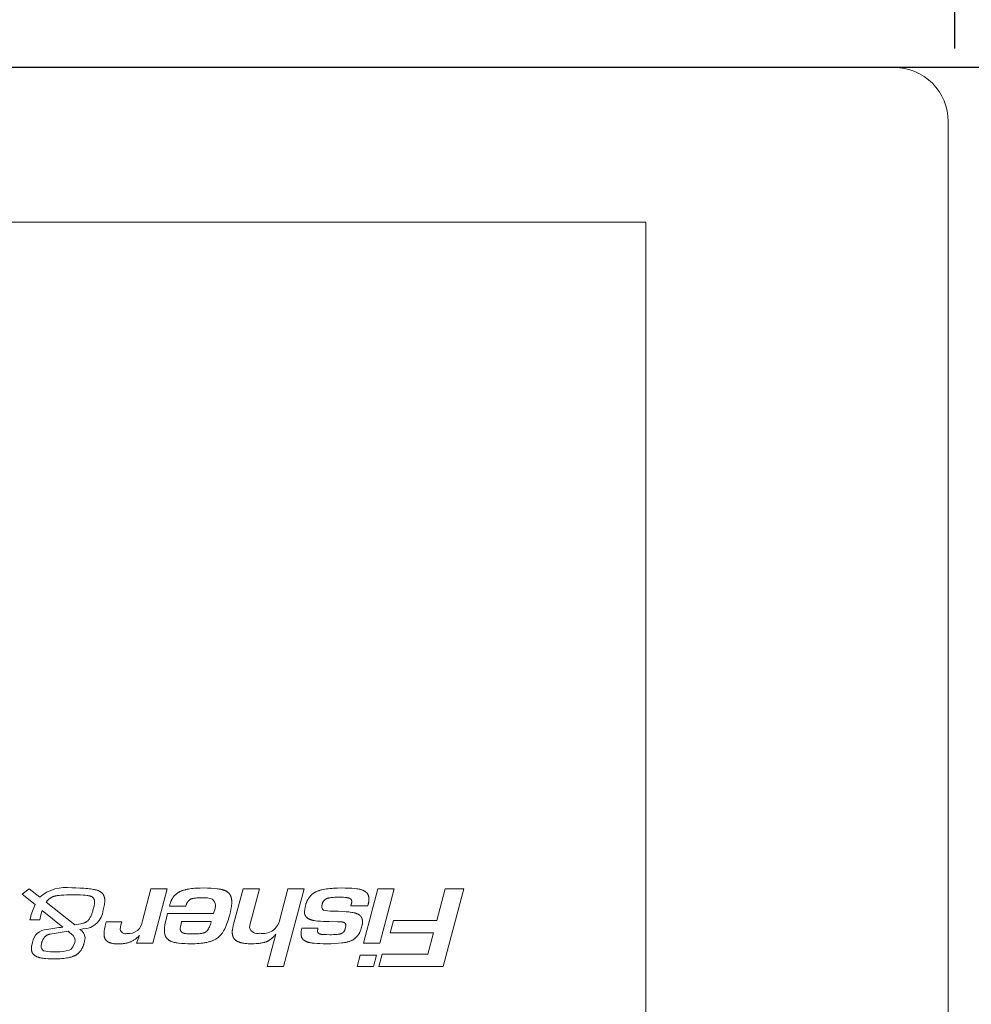
# Model space of a CAD drawing. Units: inches. Extents: x -1198 to -69, y -512 to 437.
# Tile 12 of 50: x -948.245 to -945.108, y 182.142 to 185.385. Entities that reach past the tile are written whole.
import ezdxf

# ---------------------------------------------------------------- set-up
doc = ezdxf.new("R2010")
doc.units = ezdxf.units.IN
doc.header["$MEASUREMENT"] = 0
for name, color, linetype, lineweight in [('0_Pen_No__7', 7, 'Continuous', 18), ('A-ANNO-DIMS', 2, 'Continuous', 18), ('A-EQPM', 60, 'Continuous', 18), ('A-FLOR-CASE', 7, 'Continuous', 25)]:
    doc.layers.add(name, color=color, linetype=linetype, lineweight=lineweight)
doc.styles.get("Standard").update_dxf_attribs({"font": 'arial.ttf'})
doc.dimstyles.get("Standard").update_dxf_attribs({"dimtxt": 6, "dimasz": 6, "dimexe": 0.18, "dimexo": 0.0625, "dimgap": 0.09, "dimtad": 0, "dimtih": 1, "dimtoh": 1, "dimdec": 0, "dimzin": 0, "dimdsep": 46, "dimlunit": 4, "dimtxsty": 'Standard', "dimblk": 'OBLIQUE', "dimcen": 0.09, "dimadec": 0, "dimazin": 0, "dimtfac": 1, "dimtdec": 0, "dimtofl": 0, "dimtmove": 0, "dimatfit": 3, "dimfxl": 1, "dimtolj": 1, "dimtzin": 0, "dimarcsym": 0})

# ---------------------------------------------------------------- blocks, each defined once
blk = doc.blocks.new('new block')
at = {"layer": '0_Pen_No__7'}
for p, q in [((-318.452, 68.7), (-316.721, 75.2)), ((-316.721, 75.2), (-311.349, 75.2)), ((-311.349, 75.2), (-311.629, 74.168)), ((-311.16, 74.266), (-310.904, 75.2)), ((-310.904, 75.2), (-309.527, 75.2)), ((-309.527, 75.2), (-309.782, 74.266)), ((-305.104, 68.7), (-303.373, 75.2)), ((-303.373, 75.2), (-301.997, 75.2)), ((-301.997, 75.2), (-302.715, 72.502)), ((-315.442, 74.168), (-315.906, 72.403)), ((-311.629, 74.168), (-315.442, 74.168)), ((-309.782, 74.266), (-311.16, 74.266)), ((-312.634, 68.7), (-311.429, 73.251)), ((-311.429, 73.251), (-310.05, 73.251)), ((-310.05, 73.251), (-311.257, 68.7)), ((-293.639, 68.7), (-292.433, 73.251)), ((-292.433, 73.251), (-291.056, 73.251)), ((-291.056, 73.251), (-291.311, 72.618)), ((-286.771, 72.786), (-286.716, 73.132)), ((-285.755, 72.627), (-285.462, 72.368)), ((-315.906, 72.403), (-312.288, 72.403)), ((-312.288, 72.403), (-312.567, 71.371)), ((-306.237, 72.004), (-306.225, 72.092)), ((-304.908, 72.004), (-306.237, 72.004)), ((-306.225, 72.092), (-306.213, 72.219)), ((-300.571, 71.634), (-300.522, 71.955)), ((-299.158, 71.789), (-299.974, 68.7)), ((-294.784, 71.634), (-294.723, 72.033)), ((-289.824, 71.488), (-289.753, 71.731)), ((-289.753, 71.731), (-289.691, 72.102)), ((-288.448, 71.819), (-288.533, 71.488)), ((-286.562, 72.059), (-286.329, 72.102)), ((-283.509, 69.837), (-285.894, 71.738)), ((-285.462, 72.368), (-285.335, 72.264)), ((-284.895, 71.907), (-283.174, 70.513)), ((-316.186, 71.371), (-316.892, 68.7)), ((-312.567, 71.371), (-316.186, 71.371)), ((-303.045, 71.283), (-303.727, 68.7)), ((-301.351, 68.7), (-300.571, 71.634)), ((-297.319, 71.458), (-294.833, 71.458)), ((-294.833, 71.458), (-294.784, 71.634)), ((-293.566, 71.146), (-293.663, 70.776)), ((-291.555, 71.379), (-292.26, 68.7)), ((-288.533, 71.488), (-289.824, 71.488)), ((-283.174, 70.513), (-283.064, 70.877)), ((-283.064, 70.877), (-282.962, 71.312)), ((-282.962, 71.312), (-282.141, 71.312)), ((-282.242, 70.858), (-282.564, 70.016)), ((-282.174, 71.152), (-282.242, 70.858)), ((-282.141, 71.312), (-282.174, 71.152)), ((-310.452, 70.006), (-310.417, 70.134)), ((-310.417, 70.134), (-309.003, 70.134)), ((-309.003, 70.134), (-309.04, 69.986)), ((-306.725, 70.503), (-307.261, 70.58)), ((-305.117, 70.62), (-305.202, 70.114)), ((-297.514, 70.776), (-297.561, 70.601)), ((-293.663, 70.776), (-297.514, 70.776)), ((-295.187, 70.152), (-293.822, 70.152)), ((-293.846, 70.065), (-293.858, 70.016)), ((-293.822, 70.152), (-293.846, 70.065)), ((-288.382, 70.016), (-288.272, 70.467)), ((-288.405, 69.686), (-288.382, 70.016)), ((-282.063, 68.7), (-282.973, 69.42)), ((-282.564, 70.016), (-281.486, 69.163)), ((-316.892, 68.7), (-318.452, 68.7)), ((-311.257, 68.7), (-312.634, 68.7)), ((-303.727, 68.7), (-305.104, 68.7)), ((-299.974, 68.7), (-301.351, 68.7)), ((-292.26, 68.7), (-293.639, 68.7)), ((-281.486, 69.163), (-282.063, 68.7))]:
    blk.add_line(p, q, dxfattribs=at)
blk.add_lwpolyline([(-354.492, 596.906), (481.176, 596.906, -0.414214), (485.681, 592.401), (485.681, 99.109), (486.244, 99.109), (486.244, 95.73), (485.681, 95.73), (485.681, 4.505, -0.414214), (481.176, 0), (-354.492, 0, -0.414214), (-358.997, 4.505), (-358.997, 95.73), (-359.56, 95.73), (-359.56, 99.109), (-358.997, 99.109), (-358.997, 592.401, -0.414214)], format="xyb", close=True, dxfattribs=at)
blk.add_lwpolyline([(-333.701, 12.952), (460.296, 12.952), (460.296, 570.439), (-333.701, 570.439)], close=True, dxfattribs=at)
for points in [[(-286.716, 73.132), (-286.69, 73.224), (-286.662, 73.317), (-286.646, 73.362), (-286.63, 73.408), (-286.613, 73.453), (-286.595, 73.498), (-286.577, 73.543), (-286.557, 73.587), (-286.536, 73.63), (-286.514, 73.673), (-286.492, 73.716), (-286.468, 73.757), (-286.443, 73.799), (-286.417, 73.839), (-286.394, 73.873), (-286.37, 73.906), (-286.345, 73.938), (-286.32, 73.97), (-286.294, 74.001), (-286.266, 74.031), (-286.238, 74.06), (-286.209, 74.089), (-286.181, 74.115), (-286.152, 74.14), (-286.122, 74.164), (-286.091, 74.187), (-286.06, 74.209), (-286.028, 74.23), (-285.996, 74.25), (-285.963, 74.269), (-285.924, 74.29), (-285.885, 74.309), (-285.846, 74.327), (-285.806, 74.344), (-285.765, 74.36), (-285.724, 74.375), (-285.683, 74.389), (-285.641, 74.402), (-285.59, 74.417), (-285.538, 74.431), (-285.486, 74.444), (-285.434, 74.456), (-285.329, 74.478), (-285.223, 74.496), (-285.084, 74.517), (-284.943, 74.534), (-284.803, 74.547), (-284.662, 74.557), (-284.521, 74.564), (-284.379, 74.568), (-284.097, 74.572)], [(-284.097, 74.572), (-283.885, 74.569), (-283.673, 74.56), (-283.461, 74.545), (-283.355, 74.535), (-283.249, 74.523), (-283.177, 74.513), (-283.105, 74.502), (-283.033, 74.489), (-282.997, 74.481), (-282.962, 74.473), (-282.926, 74.464), (-282.891, 74.455), (-282.856, 74.444), (-282.821, 74.433), (-282.787, 74.42), (-282.753, 74.407), (-282.719, 74.393), (-282.686, 74.377), (-282.662, 74.365), (-282.639, 74.353), (-282.616, 74.34), (-282.594, 74.326), (-282.572, 74.312), (-282.55, 74.297), (-282.529, 74.282), (-282.508, 74.266), (-282.488, 74.249), (-282.478, 74.24), (-282.469, 74.232), (-282.459, 74.223), (-282.45, 74.214), (-282.441, 74.204), (-282.432, 74.195), (-282.423, 74.186), (-282.415, 74.176), (-282.407, 74.166), (-282.399, 74.156), (-282.391, 74.146), (-282.383, 74.135), (-282.376, 74.125), (-282.369, 74.114), (-282.362, 74.103), (-282.355, 74.091), (-282.349, 74.08), (-282.343, 74.068), (-282.337, 74.056), (-282.331, 74.044), (-282.326, 74.032), (-282.32, 74.02), (-282.315, 74.007), (-282.311, 73.995), (-282.306, 73.982), (-282.302, 73.969), (-282.298, 73.956), (-282.294, 73.943), (-282.291, 73.93), (-282.288, 73.917), (-282.282, 73.891), (-282.277, 73.864), (-282.273, 73.837), (-282.269, 73.81), (-282.267, 73.782), (-282.265, 73.755), (-282.264, 73.728), (-282.263, 73.701), (-282.263, 73.669), (-282.265, 73.638), (-282.267, 73.606), (-282.269, 73.575), (-282.273, 73.544), (-282.277, 73.513), (-282.282, 73.482), (-282.287, 73.451), (-282.299, 73.39), (-282.312, 73.329), (-282.342, 73.207)], [(-291.311, 72.618), (-291.264, 72.662), (-291.217, 72.706), (-291.168, 72.749), (-291.119, 72.792), (-291.069, 72.833), (-291.018, 72.873), (-290.966, 72.911), (-290.913, 72.949), (-290.866, 72.98), (-290.819, 73.011), (-290.771, 73.04), (-290.722, 73.068), (-290.673, 73.094), (-290.623, 73.119), (-290.572, 73.142), (-290.521, 73.164), (-290.468, 73.184), (-290.414, 73.203), (-290.359, 73.219), (-290.304, 73.235), (-290.249, 73.248), (-290.193, 73.26), (-290.137, 73.271), (-290.081, 73.281), (-290.017, 73.29), (-289.953, 73.298), (-289.889, 73.304), (-289.825, 73.31), (-289.755, 73.314), (-289.685, 73.317), (-289.545, 73.319), (-289.472, 73.319), (-289.4, 73.317), (-289.327, 73.313), (-289.255, 73.307), (-289.192, 73.301), (-289.13, 73.293), (-289.068, 73.283), (-289.006, 73.271), (-288.956, 73.26), (-288.907, 73.247), (-288.883, 73.24), (-288.859, 73.233), (-288.835, 73.225), (-288.811, 73.216), (-288.787, 73.207), (-288.764, 73.197), (-288.741, 73.187), (-288.718, 73.176), (-288.696, 73.164), (-288.674, 73.151), (-288.663, 73.145), (-288.653, 73.138), (-288.642, 73.131), (-288.632, 73.124), (-288.615, 73.111), (-288.598, 73.098), (-288.581, 73.085), (-288.565, 73.07), (-288.549, 73.056), (-288.534, 73.041), (-288.52, 73.025), (-288.505, 73.009), (-288.492, 72.992), (-288.478, 72.975), (-288.466, 72.958), (-288.454, 72.94), (-288.442, 72.922), (-288.432, 72.904), (-288.422, 72.885), (-288.412, 72.866), (-288.407, 72.855), (-288.402, 72.844), (-288.397, 72.832), (-288.393, 72.821), (-288.389, 72.81), (-288.385, 72.798), (-288.381, 72.786), (-288.377, 72.775), (-288.37, 72.751), (-288.364, 72.727), (-288.359, 72.703), (-288.355, 72.679), (-288.351, 72.654), (-288.347, 72.63), (-288.345, 72.605), (-288.343, 72.58), (-288.341, 72.556), (-288.34, 72.531), (-288.339, 72.481), (-288.34, 72.439), (-288.341, 72.396), (-288.344, 72.354), (-288.347, 72.312), (-288.352, 72.27), (-288.357, 72.229), (-288.363, 72.187), (-288.37, 72.145), (-288.386, 72.063), (-288.405, 71.981), (-288.426, 71.9), (-288.448, 71.819)], [(-285.335, 72.264), (-283.828, 72.5), (-283.806, 72.504), (-283.784, 72.508), (-283.762, 72.514), (-283.739, 72.519), (-283.717, 72.526), (-283.695, 72.533), (-283.673, 72.541), (-283.652, 72.549), (-283.631, 72.558), (-283.609, 72.567), (-283.59, 72.577), (-283.572, 72.587), (-283.553, 72.597), (-283.535, 72.608), (-283.517, 72.62), (-283.5, 72.632), (-283.483, 72.644), (-283.466, 72.657), (-283.45, 72.67), (-283.435, 72.684), (-283.42, 72.697), (-283.405, 72.712), (-283.391, 72.726), (-283.377, 72.741), (-283.364, 72.756), (-283.351, 72.772), (-283.338, 72.787), (-283.326, 72.804), (-283.313, 72.82), (-283.302, 72.837), (-283.29, 72.853), (-283.279, 72.871), (-283.268, 72.888), (-283.258, 72.905), (-283.248, 72.923), (-283.239, 72.94), (-283.22, 72.976), (-283.204, 73.012), (-283.188, 73.049), (-283.173, 73.086), (-283.159, 73.123), (-283.146, 73.161), (-283.134, 73.199), (-283.124, 73.235), (-283.115, 73.27), (-283.097, 73.342), (-283.082, 73.414), (-283.068, 73.487)], [(-309.904, 71.926), (-309.878, 72.017), (-309.864, 72.062), (-309.849, 72.107), (-309.833, 72.152), (-309.816, 72.196), (-309.798, 72.24), (-309.78, 72.283), (-309.76, 72.326), (-309.739, 72.369), (-309.717, 72.411), (-309.694, 72.452), (-309.67, 72.493), (-309.645, 72.533), (-309.618, 72.572), (-309.591, 72.61), (-309.566, 72.643), (-309.54, 72.676), (-309.512, 72.707), (-309.484, 72.738), (-309.455, 72.768), (-309.426, 72.797), (-309.395, 72.825), (-309.363, 72.852), (-309.331, 72.878), (-309.298, 72.902), (-309.265, 72.926), (-309.23, 72.948), (-309.196, 72.969), (-309.16, 72.99), (-309.124, 73.009), (-309.087, 73.027), (-309.039, 73.05), (-308.989, 73.071), (-308.939, 73.091), (-308.888, 73.108), (-308.837, 73.125), (-308.785, 73.14), (-308.732, 73.154), (-308.68, 73.167), (-308.627, 73.179), (-308.573, 73.19), (-308.466, 73.209), (-308.359, 73.225), (-308.251, 73.239), (-307.955, 73.271), (-307.661, 73.292), (-307.323, 73.305), (-306.956, 73.31), (-306.678, 73.308), (-306.4, 73.299), (-306.169, 73.285), (-305.939, 73.266), (-305.777, 73.248), (-305.696, 73.237), (-305.615, 73.224), (-305.575, 73.216), (-305.535, 73.207), (-305.496, 73.198), (-305.456, 73.188), (-305.416, 73.176), (-305.377, 73.164), (-305.338, 73.15), (-305.299, 73.135), (-305.274, 73.124), (-305.249, 73.113), (-305.224, 73.102), (-305.199, 73.09), (-305.175, 73.077), (-305.151, 73.063), (-305.128, 73.049), (-305.105, 73.034), (-305.094, 73.026), (-305.083, 73.019), (-305.072, 73.01), (-305.062, 73.002), (-305.051, 72.994), (-305.041, 72.985), (-305.031, 72.976), (-305.021, 72.967), (-305.011, 72.958), (-305.002, 72.949), (-304.993, 72.939), (-304.984, 72.929), (-304.975, 72.919), (-304.967, 72.909), (-304.959, 72.899), (-304.951, 72.888), (-304.944, 72.877), (-304.937, 72.866), (-304.93, 72.855), (-304.923, 72.844), (-304.917, 72.832), (-304.911, 72.821), (-304.905, 72.809), (-304.899, 72.797), (-304.894, 72.785), (-304.889, 72.772), (-304.884, 72.76), (-304.88, 72.747), (-304.875, 72.735), (-304.871, 72.722), (-304.868, 72.709), (-304.864, 72.696), (-304.861, 72.683), (-304.858, 72.67), (-304.852, 72.643), (-304.847, 72.616), (-304.843, 72.589), (-304.84, 72.562), (-304.838, 72.535), (-304.837, 72.508), (-304.836, 72.481), (-304.836, 72.45), (-304.836, 72.42), (-304.838, 72.389), (-304.84, 72.359), (-304.843, 72.329), (-304.847, 72.299), (-304.852, 72.269), (-304.856, 72.239), (-304.867, 72.18), (-304.88, 72.121), (-304.908, 72.004)], [(-307.236, 72.55), (-307.388, 72.549), (-307.54, 72.544), (-307.693, 72.536), (-307.846, 72.525), (-307.939, 72.516), (-307.986, 72.511), (-308.009, 72.507), (-308.032, 72.503), (-308.055, 72.499), (-308.078, 72.494), (-308.101, 72.489), (-308.123, 72.483), (-308.145, 72.476), (-308.167, 72.469), (-308.189, 72.461), (-308.2, 72.457), (-308.211, 72.452), (-308.224, 72.446), (-308.238, 72.44), (-308.251, 72.433), (-308.264, 72.426), (-308.277, 72.418), (-308.29, 72.411), (-308.302, 72.403), (-308.315, 72.394), (-308.327, 72.386), (-308.338, 72.377), (-308.35, 72.367), (-308.361, 72.358), (-308.372, 72.348), (-308.383, 72.337), (-308.393, 72.326), (-308.403, 72.315), (-308.413, 72.304), (-308.422, 72.292), (-308.431, 72.28), (-308.439, 72.267), (-308.447, 72.255), (-308.455, 72.242), (-308.463, 72.228), (-308.47, 72.215), (-308.477, 72.201), (-308.483, 72.188), (-308.489, 72.174), (-308.495, 72.159), (-308.5, 72.145), (-308.505, 72.131), (-308.51, 72.117), (-308.515, 72.102), (-308.522, 72.075), (-308.529, 72.048), (-308.535, 72.02), (-308.568, 71.844), (-308.572, 71.825), (-308.575, 71.807), (-308.577, 71.788), (-308.578, 71.769), (-308.578, 71.75), (-308.577, 71.736), (-308.576, 71.721), (-308.574, 71.711), (-308.572, 71.701), (-308.57, 71.691), (-308.567, 71.681), (-308.564, 71.671), (-308.561, 71.662), (-308.557, 71.652), (-308.552, 71.643), (-308.548, 71.634), (-308.543, 71.625), (-308.538, 71.616), (-308.532, 71.608), (-308.526, 71.6), (-308.516, 71.589), (-308.508, 71.58), (-308.499, 71.572), (-308.489, 71.563), (-308.478, 71.556), (-308.467, 71.549), (-308.455, 71.542), (-308.444, 71.536), (-308.431, 71.531), (-308.413, 71.523), (-308.4, 71.519), (-308.387, 71.514), (-308.374, 71.511), (-308.36, 71.507), (-308.347, 71.504), (-308.32, 71.498), (-308.294, 71.493), (-308.268, 71.488), (-308.243, 71.484), (-308.217, 71.48), (-308.166, 71.474), (-308.115, 71.47), (-308.064, 71.466), (-307.913, 71.461), (-307.2, 71.448)], [(-306.213, 72.219), (-306.213, 72.23), (-306.213, 72.242), (-306.214, 72.253), (-306.215, 72.265), (-306.217, 72.277), (-306.219, 72.288), (-306.221, 72.3), (-306.224, 72.311), (-306.227, 72.322), (-306.23, 72.333), (-306.234, 72.344), (-306.239, 72.354), (-306.244, 72.365), (-306.249, 72.375), (-306.255, 72.384), (-306.261, 72.394), (-306.268, 72.402), (-306.275, 72.411), (-306.283, 72.419), (-306.291, 72.426), (-306.299, 72.433), (-306.308, 72.44), (-306.317, 72.447), (-306.326, 72.453), (-306.336, 72.459), (-306.346, 72.465), (-306.356, 72.47), (-306.366, 72.475), (-306.376, 72.48), (-306.387, 72.484), (-306.397, 72.488), (-306.408, 72.492), (-306.427, 72.498), (-306.445, 72.504), (-306.464, 72.509), (-306.483, 72.513), (-306.502, 72.517), (-306.521, 72.52), (-306.54, 72.523), (-306.559, 72.526), (-306.597, 72.529), (-306.635, 72.532), (-306.974, 72.546), (-307.236, 72.55)], [(-302.715, 72.502), (-302.674, 72.555), (-302.631, 72.607), (-302.588, 72.659), (-302.542, 72.709), (-302.495, 72.757), (-302.447, 72.804), (-302.422, 72.827), (-302.396, 72.85), (-302.371, 72.872), (-302.345, 72.893), (-302.321, 72.912), (-302.298, 72.93), (-302.274, 72.947), (-302.249, 72.965), (-302.225, 72.981), (-302.2, 72.998), (-302.175, 73.014), (-302.149, 73.029), (-302.124, 73.044), (-302.098, 73.059), (-302.072, 73.073), (-302.045, 73.086), (-302.018, 73.099), (-301.991, 73.112), (-301.964, 73.124), (-301.937, 73.135), (-301.905, 73.147), (-301.873, 73.159), (-301.841, 73.17), (-301.809, 73.181), (-301.776, 73.191), (-301.743, 73.2), (-301.677, 73.217), (-301.611, 73.231), (-301.544, 73.244), (-301.476, 73.256), (-301.409, 73.266), (-301.327, 73.277), (-301.244, 73.286), (-301.162, 73.293), (-301.079, 73.299), (-300.893, 73.307), (-300.706, 73.31), (-300.505, 73.307), (-300.404, 73.302), (-300.304, 73.296), (-300.218, 73.288), (-300.133, 73.279), (-300.048, 73.267), (-299.963, 73.254), (-299.897, 73.241), (-299.833, 73.227), (-299.8, 73.22), (-299.768, 73.211), (-299.736, 73.202), (-299.705, 73.193), (-299.673, 73.182), (-299.642, 73.171), (-299.611, 73.159), (-299.581, 73.146), (-299.551, 73.133), (-299.521, 73.118), (-299.492, 73.102), (-299.477, 73.094), (-299.463, 73.085), (-299.441, 73.071), (-299.419, 73.057), (-299.397, 73.041), (-299.376, 73.025), (-299.356, 73.009), (-299.335, 72.992), (-299.316, 72.974), (-299.297, 72.955), (-299.278, 72.936), (-299.261, 72.917), (-299.244, 72.897), (-299.236, 72.887), (-299.228, 72.876), (-299.22, 72.866), (-299.212, 72.855), (-299.205, 72.844), (-299.197, 72.833), (-299.19, 72.822), (-299.184, 72.811), (-299.177, 72.8), (-299.171, 72.788), (-299.164, 72.776), (-299.158, 72.763), (-299.152, 72.751), (-299.146, 72.738), (-299.14, 72.725), (-299.135, 72.712), (-299.13, 72.698), (-299.125, 72.685), (-299.121, 72.672), (-299.116, 72.658), (-299.109, 72.631), (-299.101, 72.603), (-299.095, 72.575), (-299.09, 72.547), (-299.085, 72.518), (-299.082, 72.49), (-299.079, 72.461), (-299.076, 72.433), (-299.075, 72.404), (-299.074, 72.375), (-299.073, 72.346), (-299.073, 72.311), (-299.074, 72.275), (-299.076, 72.239), (-299.079, 72.204), (-299.082, 72.169), (-299.086, 72.134), (-299.091, 72.099), (-299.096, 72.064), (-299.109, 71.994), (-299.123, 71.925), (-299.14, 71.857), (-299.158, 71.789)], [(-298.842, 70.97), (-298.801, 71.12), (-298.757, 71.27), (-298.71, 71.418), (-298.659, 71.565), (-298.603, 71.711), (-298.574, 71.783), (-298.543, 71.854), (-298.511, 71.925), (-298.477, 71.995), (-298.442, 72.064), (-298.406, 72.133), (-298.376, 72.186), (-298.345, 72.239), (-298.313, 72.292), (-298.28, 72.343), (-298.246, 72.394), (-298.211, 72.444), (-298.174, 72.493), (-298.135, 72.54), (-298.101, 72.581), (-298.066, 72.62), (-298.029, 72.659), (-297.992, 72.696), (-297.953, 72.733), (-297.913, 72.767), (-297.893, 72.784), (-297.872, 72.801), (-297.851, 72.817), (-297.83, 72.833), (-297.808, 72.849), (-297.785, 72.864), (-297.763, 72.879), (-297.739, 72.894), (-297.692, 72.922), (-297.645, 72.948), (-297.596, 72.974), (-297.546, 72.997), (-297.496, 73.02), (-297.446, 73.041), (-297.385, 73.064), (-297.324, 73.086), (-297.263, 73.107), (-297.201, 73.126), (-297.139, 73.144), (-297.076, 73.16), (-296.95, 73.19), (-296.869, 73.207), (-296.787, 73.222), (-296.705, 73.236), (-296.622, 73.249), (-296.457, 73.27), (-296.291, 73.286), (-296.125, 73.297), (-295.958, 73.305), (-295.625, 73.31)], [(-295.807, 72.492), (-295.973, 72.49), (-296.056, 72.488), (-296.139, 72.484), (-296.222, 72.478), (-296.304, 72.47), (-296.386, 72.46), (-296.468, 72.448), (-296.526, 72.437), (-296.585, 72.424), (-296.614, 72.417), (-296.643, 72.41), (-296.671, 72.401), (-296.7, 72.392), (-296.722, 72.385), (-296.744, 72.377), (-296.765, 72.369), (-296.787, 72.36), (-296.797, 72.355), (-296.808, 72.35), (-296.818, 72.345), (-296.828, 72.339), (-296.838, 72.334), (-296.848, 72.328), (-296.858, 72.322), (-296.867, 72.315), (-296.876, 72.309), (-296.885, 72.303), (-296.893, 72.296), (-296.902, 72.29), (-296.91, 72.283), (-296.918, 72.275), (-296.926, 72.268), (-296.934, 72.261), (-296.941, 72.253), (-296.949, 72.245), (-296.964, 72.229), (-296.978, 72.213), (-296.992, 72.196), (-297.008, 72.175), (-297.024, 72.153), (-297.04, 72.13), (-297.054, 72.107), (-297.069, 72.084), (-297.082, 72.061), (-297.109, 72.013), (-297.126, 71.98), (-297.142, 71.947), (-297.158, 71.913), (-297.173, 71.879), (-297.201, 71.811), (-297.228, 71.741), (-297.253, 71.671), (-297.276, 71.6), (-297.319, 71.458)], [(-294.723, 72.033), (-294.723, 72.048), (-294.724, 72.063), (-294.725, 72.079), (-294.726, 72.094), (-294.728, 72.11), (-294.73, 72.125), (-294.732, 72.14), (-294.736, 72.155), (-294.739, 72.17), (-294.743, 72.185), (-294.748, 72.2), (-294.753, 72.214), (-294.759, 72.228), (-294.766, 72.242), (-294.773, 72.255), (-294.781, 72.268), (-294.789, 72.279), (-294.797, 72.29), (-294.806, 72.3), (-294.815, 72.31), (-294.825, 72.32), (-294.835, 72.329), (-294.846, 72.338), (-294.857, 72.347), (-294.868, 72.355), (-294.88, 72.363), (-294.891, 72.37), (-294.904, 72.377), (-294.916, 72.384), (-294.928, 72.391), (-294.941, 72.397), (-294.954, 72.403), (-294.963, 72.407), (-294.973, 72.411), (-294.992, 72.418), (-295.012, 72.425), (-295.032, 72.431), (-295.052, 72.436), (-295.072, 72.441), (-295.092, 72.445), (-295.113, 72.449), (-295.133, 72.453), (-295.154, 72.456), (-295.195, 72.461), (-295.277, 72.469), (-295.41, 72.479), (-295.542, 72.486), (-295.675, 72.491), (-295.807, 72.492)], [(-295.625, 73.31), (-295.36, 73.306), (-295.094, 73.296), (-294.828, 73.278), (-294.562, 73.251), (-294.474, 73.241), (-294.386, 73.229), (-294.299, 73.214), (-294.255, 73.205), (-294.212, 73.196), (-294.169, 73.186), (-294.127, 73.174), (-294.085, 73.161), (-294.043, 73.147), (-294.002, 73.132), (-293.982, 73.124), (-293.962, 73.115), (-293.942, 73.106), (-293.922, 73.097), (-293.902, 73.087), (-293.882, 73.077), (-293.855, 73.062), (-293.827, 73.045), (-293.8, 73.028), (-293.774, 73.01), (-293.748, 72.991), (-293.723, 72.972), (-293.699, 72.951), (-293.675, 72.93), (-293.652, 72.908), (-293.641, 72.897), (-293.63, 72.886), (-293.619, 72.874), (-293.608, 72.862), (-293.598, 72.85), (-293.588, 72.838), (-293.578, 72.826), (-293.568, 72.813), (-293.559, 72.801), (-293.55, 72.788), (-293.541, 72.775), (-293.533, 72.762), (-293.525, 72.748), (-293.517, 72.735), (-293.508, 72.719), (-293.5, 72.704), (-293.492, 72.688), (-293.484, 72.672), (-293.477, 72.655), (-293.47, 72.639), (-293.464, 72.622), (-293.458, 72.606), (-293.452, 72.589), (-293.447, 72.572), (-293.442, 72.555), (-293.437, 72.537), (-293.432, 72.52), (-293.428, 72.503), (-293.42, 72.467), (-293.414, 72.432), (-293.409, 72.396), (-293.404, 72.36), (-293.401, 72.324), (-293.398, 72.288), (-293.396, 72.251), (-293.395, 72.215), (-293.395, 72.179), (-293.396, 72.122), (-293.398, 72.065), (-293.402, 72.009), (-293.407, 71.953), (-293.413, 71.897), (-293.42, 71.842), (-293.437, 71.731), (-293.464, 71.584), (-293.495, 71.437), (-293.529, 71.291), (-293.566, 71.146)], [(-307.261, 70.58), (-307.93, 70.588), (-308.264, 70.602), (-308.598, 70.625), (-308.835, 70.648), (-308.954, 70.663), (-309.072, 70.68), (-309.159, 70.695), (-309.246, 70.712), (-309.29, 70.722), (-309.333, 70.732), (-309.375, 70.744), (-309.418, 70.757), (-309.45, 70.767), (-309.481, 70.779), (-309.513, 70.791), (-309.543, 70.804), (-309.574, 70.818), (-309.604, 70.833), (-309.619, 70.841), (-309.634, 70.849), (-309.648, 70.857), (-309.663, 70.866), (-309.675, 70.874), (-309.687, 70.882), (-309.699, 70.89), (-309.711, 70.898), (-309.723, 70.907), (-309.734, 70.916), (-309.746, 70.925), (-309.757, 70.934), (-309.768, 70.944), (-309.778, 70.954), (-309.789, 70.964), (-309.799, 70.974), (-309.809, 70.984), (-309.819, 70.995), (-309.828, 71.006), (-309.837, 71.017), (-309.846, 71.029), (-309.854, 71.04), (-309.862, 71.052), (-309.87, 71.064), (-309.877, 71.076), (-309.884, 71.088), (-309.891, 71.101), (-309.898, 71.113), (-309.904, 71.126), (-309.91, 71.139), (-309.916, 71.152), (-309.921, 71.165), (-309.926, 71.179), (-309.931, 71.192), (-309.936, 71.206), (-309.94, 71.22), (-309.944, 71.234), (-309.948, 71.248), (-309.952, 71.262), (-309.955, 71.276), (-309.961, 71.304), (-309.966, 71.333), (-309.97, 71.362), (-309.973, 71.39), (-309.976, 71.419), (-309.977, 71.448), (-309.977, 71.479), (-309.977, 71.509), (-309.976, 71.54), (-309.973, 71.57), (-309.97, 71.6), (-309.967, 71.63), (-309.963, 71.66), (-309.958, 71.69), (-309.946, 71.75), (-309.933, 71.809), (-309.904, 71.926)], [(-285.894, 71.738), (-286.234, 71.675), (-286.403, 71.638), (-286.486, 71.617), (-286.57, 71.594), (-286.625, 71.577), (-286.679, 71.559), (-286.706, 71.549), (-286.733, 71.539), (-286.76, 71.528), (-286.786, 71.517), (-286.806, 71.507), (-286.826, 71.497), (-286.846, 71.487), (-286.865, 71.476), (-286.884, 71.465), (-286.893, 71.459), (-286.902, 71.453), (-286.911, 71.447), (-286.92, 71.44), (-286.929, 71.434), (-286.937, 71.427), (-286.946, 71.42), (-286.955, 71.412), (-286.963, 71.405), (-286.971, 71.397), (-286.979, 71.389), (-286.987, 71.381), (-287.003, 71.364), (-287.018, 71.347), (-287.032, 71.329), (-287.046, 71.311), (-287.06, 71.293), (-287.078, 71.268), (-287.095, 71.243), (-287.112, 71.218), (-287.128, 71.193), (-287.159, 71.142), (-287.188, 71.09), (-287.207, 71.055), (-287.225, 71.02), (-287.258, 70.949), (-287.29, 70.876), (-287.32, 70.803), (-287.347, 70.729), (-287.372, 70.654), (-287.396, 70.579), (-287.417, 70.503)], [(-307.2, 71.448), (-306.952, 71.446), (-306.705, 71.438), (-306.457, 71.425), (-306.209, 71.405), (-306.049, 71.387), (-305.969, 71.376), (-305.89, 71.363), (-305.851, 71.355), (-305.811, 71.347), (-305.772, 71.337), (-305.733, 71.327), (-305.694, 71.315), (-305.656, 71.303), (-305.617, 71.289), (-305.579, 71.274), (-305.554, 71.263), (-305.529, 71.252), (-305.504, 71.24), (-305.48, 71.228), (-305.455, 71.215), (-305.432, 71.201), (-305.409, 71.187), (-305.386, 71.171), (-305.375, 71.164), (-305.364, 71.156), (-305.353, 71.147), (-305.342, 71.139), (-305.332, 71.13), (-305.322, 71.122), (-305.312, 71.113), (-305.302, 71.103), (-305.292, 71.094), (-305.283, 71.084), (-305.274, 71.075), (-305.265, 71.065), (-305.256, 71.055), (-305.248, 71.044), (-305.24, 71.034), (-305.232, 71.023), (-305.225, 71.012), (-305.217, 71.001), (-305.211, 70.99), (-305.204, 70.978), (-305.198, 70.967), (-305.191, 70.955), (-305.186, 70.943), (-305.18, 70.931), (-305.175, 70.919), (-305.17, 70.907), (-305.165, 70.895), (-305.16, 70.882), (-305.156, 70.87), (-305.152, 70.857), (-305.148, 70.844), (-305.144, 70.831), (-305.141, 70.818), (-305.138, 70.805), (-305.135, 70.792), (-305.132, 70.779), (-305.127, 70.752), (-305.123, 70.726), (-305.12, 70.699), (-305.118, 70.673), (-305.117, 70.647), (-305.117, 70.62)], [(-293.858, 70.016), (-293.869, 69.973), (-293.882, 69.929), (-293.895, 69.886), (-293.91, 69.844), (-293.925, 69.801), (-293.942, 69.759), (-293.96, 69.717), (-293.978, 69.676), (-293.998, 69.635), (-294.018, 69.595), (-294.04, 69.555), (-294.063, 69.516), (-294.087, 69.478), (-294.112, 69.441), (-294.139, 69.404), (-294.166, 69.368), (-294.193, 69.335), (-294.221, 69.303), (-294.25, 69.271), (-294.28, 69.241), (-294.311, 69.211), (-294.343, 69.182), (-294.375, 69.154), (-294.409, 69.127), (-294.443, 69.101), (-294.478, 69.076), (-294.513, 69.052), (-294.549, 69.028), (-294.586, 69.006), (-294.623, 68.985), (-294.66, 68.964), (-294.698, 68.945), (-294.746, 68.922), (-294.795, 68.9), (-294.844, 68.88), (-294.894, 68.862), (-294.944, 68.844), (-294.994, 68.828), (-295.045, 68.813), (-295.097, 68.799), (-295.148, 68.786), (-295.2, 68.774), (-295.305, 68.753), (-295.41, 68.734), (-295.515, 68.718), (-295.651, 68.699), (-295.788, 68.684), (-295.924, 68.671), (-296.06, 68.661), (-296.22, 68.653), (-296.379, 68.647), (-296.698, 68.642), (-297, 68.645), (-297.151, 68.65), (-297.301, 68.658), (-297.553, 68.677), (-297.806, 68.703), (-297.899, 68.714), (-297.992, 68.728), (-298.084, 68.743), (-298.13, 68.752), (-298.175, 68.762), (-298.221, 68.773), (-298.265, 68.785), (-298.31, 68.798), (-298.354, 68.813), (-298.398, 68.829), (-298.419, 68.837), (-298.441, 68.846), (-298.462, 68.856), (-298.483, 68.866), (-298.504, 68.876), (-298.525, 68.887), (-298.554, 68.902), (-298.583, 68.919), (-298.611, 68.937), (-298.639, 68.955), (-298.666, 68.975), (-298.692, 68.995), (-298.718, 69.016), (-298.743, 69.038), (-298.755, 69.049), (-298.767, 69.061), (-298.779, 69.072), (-298.791, 69.084), (-298.802, 69.096), (-298.813, 69.109), (-298.824, 69.121), (-298.834, 69.134), (-298.845, 69.147), (-298.855, 69.16), (-298.864, 69.173), (-298.874, 69.186), (-298.883, 69.2), (-298.892, 69.214), (-298.901, 69.228), (-298.909, 69.242), (-298.917, 69.257), (-298.925, 69.272), (-298.933, 69.288), (-298.94, 69.304), (-298.947, 69.32), (-298.954, 69.336), (-298.96, 69.352), (-298.966, 69.369), (-298.972, 69.385), (-298.978, 69.402), (-298.988, 69.435), (-298.997, 69.469), (-299.004, 69.503), (-299.012, 69.542), (-299.019, 69.582), (-299.024, 69.621), (-299.029, 69.661), (-299.032, 69.701), (-299.035, 69.741), (-299.036, 69.781), (-299.036, 69.82), (-299.035, 69.882), (-299.033, 69.943), (-299.028, 70.004), (-299.022, 70.065), (-299.015, 70.126), (-299.007, 70.187), (-298.988, 70.309), (-298.957, 70.475), (-298.922, 70.641), (-298.842, 70.97)], [(-305.202, 70.114), (-305.215, 70.067), (-305.229, 70.021), (-305.243, 69.974), (-305.259, 69.928), (-305.276, 69.882), (-305.294, 69.837), (-305.312, 69.791), (-305.332, 69.747), (-305.353, 69.703), (-305.375, 69.659), (-305.398, 69.616), (-305.422, 69.574), (-305.448, 69.532), (-305.474, 69.491), (-305.502, 69.451), (-305.531, 69.412), (-305.558, 69.377), (-305.587, 69.343), (-305.616, 69.309), (-305.647, 69.277), (-305.678, 69.245), (-305.71, 69.214), (-305.743, 69.185), (-305.777, 69.156), (-305.812, 69.128), (-305.848, 69.101), (-305.885, 69.076), (-305.922, 69.051), (-305.961, 69.028), (-305.999, 69.005), (-306.039, 68.984), (-306.079, 68.963), (-306.125, 68.942), (-306.171, 68.921), (-306.219, 68.902), (-306.266, 68.884), (-306.314, 68.867), (-306.363, 68.851), (-306.412, 68.836), (-306.461, 68.823), (-306.521, 68.806), (-306.582, 68.792), (-306.704, 68.765), (-306.827, 68.742), (-306.95, 68.722), (-307.098, 68.702), (-307.247, 68.686), (-307.396, 68.673), (-307.545, 68.662), (-307.883, 68.647), (-308.248, 68.642), (-308.538, 68.645), (-308.829, 68.654), (-309.073, 68.67), (-309.317, 68.691), (-309.494, 68.71), (-309.583, 68.722), (-309.671, 68.737), (-309.715, 68.746), (-309.758, 68.755), (-309.802, 68.766), (-309.845, 68.778), (-309.888, 68.79), (-309.93, 68.805), (-309.973, 68.82), (-310.014, 68.837), (-310.042, 68.849), (-310.069, 68.862), (-310.096, 68.875), (-310.122, 68.889), (-310.149, 68.904), (-310.174, 68.919), (-310.199, 68.936), (-310.224, 68.953), (-310.236, 68.961), (-310.248, 68.97), (-310.259, 68.979), (-310.271, 68.989), (-310.282, 68.998), (-310.293, 69.008), (-310.304, 69.018), (-310.314, 69.028), (-310.325, 69.039), (-310.335, 69.049), (-310.344, 69.06), (-310.354, 69.071), (-310.363, 69.082), (-310.372, 69.094), (-310.381, 69.105), (-310.389, 69.117), (-310.397, 69.129), (-310.405, 69.141), (-310.412, 69.153), (-310.419, 69.165), (-310.426, 69.177), (-310.432, 69.19), (-310.438, 69.202), (-310.444, 69.215), (-310.45, 69.228), (-310.455, 69.241), (-310.46, 69.254), (-310.465, 69.268), (-310.47, 69.281), (-310.474, 69.295), (-310.478, 69.308), (-310.482, 69.322), (-310.49, 69.35), (-310.496, 69.378), (-310.501, 69.406), (-310.505, 69.434), (-310.509, 69.463), (-310.512, 69.491), (-310.514, 69.52), (-310.515, 69.548), (-310.515, 69.575), (-310.515, 69.602), (-310.514, 69.629), (-310.512, 69.656), (-310.508, 69.709), (-310.502, 69.762), (-310.493, 69.824), (-310.488, 69.855), (-310.483, 69.886), (-310.476, 69.916), (-310.469, 69.947), (-310.461, 69.977), (-310.452, 70.006)], [(-296.562, 69.46), (-296.408, 69.462), (-296.254, 69.467), (-296.099, 69.477), (-296.022, 69.484), (-295.896, 69.498), (-295.848, 69.504), (-295.801, 69.513), (-295.777, 69.517), (-295.754, 69.523), (-295.731, 69.528), (-295.708, 69.535), (-295.685, 69.542), (-295.662, 69.549), (-295.64, 69.557), (-295.629, 69.562), (-295.618, 69.567), (-295.608, 69.571), (-295.597, 69.577), (-295.586, 69.582), (-295.576, 69.587), (-295.559, 69.597), (-295.543, 69.607), (-295.527, 69.617), (-295.512, 69.628), (-295.496, 69.639), (-295.481, 69.651), (-295.467, 69.664), (-295.452, 69.677), (-295.438, 69.69), (-295.425, 69.703), (-295.411, 69.717), (-295.398, 69.732), (-295.386, 69.746), (-295.374, 69.761), (-295.362, 69.777), (-295.351, 69.792), (-295.336, 69.813), (-295.323, 69.834), (-295.31, 69.855), (-295.298, 69.876), (-295.286, 69.898), (-295.275, 69.921), (-295.264, 69.943), (-295.254, 69.966), (-295.244, 69.989), (-295.235, 70.012), (-295.218, 70.058), (-295.202, 70.105), (-295.187, 70.152)], [(-287.417, 70.503), (-287.464, 70.331), (-287.506, 70.158), (-287.524, 70.07), (-287.532, 70.026), (-287.539, 69.982), (-287.544, 69.938), (-287.546, 69.915), (-287.548, 69.893), (-287.549, 69.871), (-287.55, 69.848), (-287.55, 69.825), (-287.549, 69.802), (-287.549, 69.782), (-287.547, 69.761), (-287.545, 69.74), (-287.542, 69.719), (-287.539, 69.698), (-287.535, 69.677), (-287.531, 69.657), (-287.528, 69.647), (-287.526, 69.636), (-287.523, 69.626), (-287.52, 69.616), (-287.516, 69.607), (-287.513, 69.597), (-287.509, 69.587), (-287.505, 69.578), (-287.501, 69.568), (-287.497, 69.559), (-287.493, 69.55), (-287.488, 69.54), (-287.483, 69.532), (-287.478, 69.523), (-287.473, 69.514), (-287.467, 69.505), (-287.461, 69.497), (-287.455, 69.489), (-287.443, 69.474), (-287.43, 69.459), (-287.416, 69.445), (-287.401, 69.431), (-287.386, 69.418), (-287.37, 69.406), (-287.354, 69.395), (-287.337, 69.384), (-287.327, 69.378), (-287.317, 69.373), (-287.308, 69.367), (-287.298, 69.362), (-287.287, 69.357), (-287.277, 69.352), (-287.267, 69.348), (-287.257, 69.343), (-287.236, 69.335), (-287.214, 69.328), (-287.193, 69.321), (-287.171, 69.314), (-287.142, 69.306), (-287.113, 69.3), (-287.083, 69.293), (-287.054, 69.288), (-286.994, 69.279), (-286.934, 69.271), (-286.767, 69.253), (-286.6, 69.24), (-286.36, 69.226), (-286.12, 69.219), (-285.639, 69.214)], [(-309.04, 69.986), (-309.048, 69.96), (-309.055, 69.934), (-309.062, 69.907), (-309.064, 69.894), (-309.067, 69.881), (-309.069, 69.867), (-309.072, 69.854), (-309.073, 69.84), (-309.075, 69.827), (-309.075, 69.813), (-309.076, 69.799), (-309.076, 69.786), (-309.076, 69.772), (-309.075, 69.76), (-309.074, 69.749), (-309.072, 69.737), (-309.07, 69.726), (-309.068, 69.714), (-309.066, 69.703), (-309.063, 69.692), (-309.059, 69.68), (-309.056, 69.67), (-309.051, 69.659), (-309.047, 69.648), (-309.042, 69.638), (-309.036, 69.628), (-309.031, 69.618), (-309.024, 69.609), (-309.018, 69.6), (-309.01, 69.59), (-309.001, 69.581), (-308.992, 69.572), (-308.982, 69.563), (-308.973, 69.555), (-308.962, 69.547), (-308.951, 69.54), (-308.94, 69.533), (-308.929, 69.526), (-308.917, 69.52), (-308.906, 69.514), (-308.894, 69.509), (-308.881, 69.503), (-308.869, 69.498), (-308.857, 69.494), (-308.844, 69.489), (-308.824, 69.482), (-308.803, 69.476), (-308.783, 69.471), (-308.762, 69.465), (-308.742, 69.461), (-308.721, 69.457), (-308.7, 69.453), (-308.679, 69.449), (-308.638, 69.444), (-308.596, 69.439), (-308.512, 69.432), (-308.396, 69.423), (-308.28, 69.417), (-308.142, 69.413), (-308.003, 69.412), (-307.832, 69.414), (-307.661, 69.42), (-307.519, 69.429), (-307.377, 69.441), (-307.275, 69.453), (-307.224, 69.461), (-307.199, 69.465), (-307.174, 69.47), (-307.149, 69.475), (-307.125, 69.481), (-307.1, 69.487), (-307.076, 69.494), (-307.052, 69.502), (-307.028, 69.51), (-307.004, 69.519), (-306.992, 69.524), (-306.981, 69.529), (-306.964, 69.537), (-306.948, 69.545), (-306.931, 69.554), (-306.915, 69.563), (-306.899, 69.573), (-306.884, 69.583), (-306.868, 69.594), (-306.853, 69.604), (-306.839, 69.616), (-306.824, 69.628), (-306.81, 69.64), (-306.797, 69.652), (-306.783, 69.665), (-306.771, 69.679), (-306.758, 69.692), (-306.746, 69.706), (-306.74, 69.715), (-306.733, 69.723), (-306.727, 69.731), (-306.721, 69.74), (-306.709, 69.757), (-306.698, 69.775), (-306.688, 69.793), (-306.678, 69.811), (-306.668, 69.83), (-306.659, 69.849), (-306.65, 69.868), (-306.642, 69.887), (-306.635, 69.907), (-306.628, 69.927), (-306.621, 69.946), (-306.614, 69.966), (-306.603, 70.006)], [(-285.652, 68.637), (-285.985, 68.64), (-286.317, 68.648), (-286.65, 68.664), (-286.815, 68.676), (-286.981, 68.691), (-287.101, 68.704), (-287.221, 68.72), (-287.341, 68.737), (-287.461, 68.758), (-287.551, 68.777), (-287.596, 68.787), (-287.641, 68.798), (-287.685, 68.809), (-287.729, 68.822), (-287.773, 68.836), (-287.817, 68.852), (-287.851, 68.865), (-287.884, 68.878), (-287.917, 68.893), (-287.95, 68.909), (-287.982, 68.926), (-287.998, 68.935), (-288.013, 68.944), (-288.029, 68.953), (-288.044, 68.963), (-288.059, 68.973), (-288.074, 68.983), (-288.087, 68.993), (-288.1, 69.003), (-288.113, 69.013), (-288.126, 69.023), (-288.138, 69.034), (-288.15, 69.044), (-288.162, 69.056), (-288.174, 69.067), (-288.185, 69.079), (-288.197, 69.09), (-288.208, 69.102), (-288.218, 69.115), (-288.229, 69.127), (-288.239, 69.14), (-288.249, 69.153), (-288.258, 69.166), (-288.267, 69.18), (-288.277, 69.195), (-288.285, 69.209), (-288.294, 69.224), (-288.302, 69.239), (-288.31, 69.254), (-288.317, 69.269), (-288.324, 69.285), (-288.331, 69.301), (-288.338, 69.316), (-288.344, 69.332), (-288.35, 69.348), (-288.355, 69.365), (-288.361, 69.381), (-288.365, 69.398), (-288.37, 69.414), (-288.374, 69.431), (-288.378, 69.448), (-288.386, 69.481), (-288.392, 69.515), (-288.396, 69.549), (-288.4, 69.584), (-288.403, 69.618), (-288.404, 69.652), (-288.405, 69.686)], [(-285.639, 69.214), (-285.191, 69.22), (-284.967, 69.23), (-284.743, 69.246), (-284.578, 69.262), (-284.495, 69.273), (-284.413, 69.285), (-284.35, 69.296), (-284.287, 69.308), (-284.255, 69.315), (-284.224, 69.323), (-284.193, 69.331), (-284.162, 69.34), (-284.137, 69.348), (-284.111, 69.356), (-284.086, 69.365), (-284.061, 69.375), (-284.036, 69.385), (-284.012, 69.395), (-283.987, 69.406), (-283.963, 69.418), (-283.94, 69.43), (-283.918, 69.442), (-283.895, 69.455), (-283.873, 69.468), (-283.851, 69.482), (-283.83, 69.497), (-283.809, 69.511), (-283.788, 69.527), (-283.767, 69.543), (-283.747, 69.56), (-283.727, 69.577), (-283.708, 69.594), (-283.689, 69.613), (-283.67, 69.631), (-283.652, 69.65), (-283.634, 69.67), (-283.617, 69.689), (-283.6, 69.71), (-283.583, 69.73), (-283.567, 69.751), (-283.552, 69.772), (-283.537, 69.794), (-283.523, 69.815), (-283.509, 69.837)]]:
    blk.add_lwpolyline(points, dxfattribs=at)
for centre, radius, start, end in [((-285.264, 73.054), 0.65, 145.25463, 220.99631), ((-285.125, 73.216), 0.705, 115.53732, 162.79084), ((-284.239, 68.997), 4.998, 79.64276, 103.77478), ((-283.503, 73.51), 0.436, 356.91901, 68.05296), ((-285.754, 72.959), 1.031, 189.64199, 236.13883), ((-283.634, 73.41), 1.308, 273.24586, 351.11338), ((-301.668, 71.062), 1.395, 77.4021, 170.88599), ((-301.171, 71.779), 0.672, 15.22031, 106.60136), ((-290.392, 71.293), 1.166, 83.68162, 175.75797), ((-290.137, 72.017), 0.454, 10.86555, 106.28223), ((-286.56, 70.341), 1.717, 90.06134, 175.7929), ((-278.463, 32.809), 39.624, 97.39024, 99.34153), ((-306.942, 70.187), 0.384, 332.01224, 55.5965), ((-296.818, 70.185), 0.852, 150.76729, 225.46616), ((-296.683, 71.747), 2.29, 251.35459, 273.04349), ((-285.137, 71.848), 3.252, 260.88312, 311.69618)]:
    blk.add_arc(centre, radius, start, end, dxfattribs=at)
blk = doc.blocks.new('COUNTER-L')
at = {"ltscale": 10}
blk.add_line((49.3491, 23.9997), (0.0001, 23.9997), dxfattribs=at)
blk = doc.blocks.new('_Oblique')
at = {"color": 0, "linetype": 'ByBlock', "lineweight": -2}
blk.add_line((-0.5, -0.5), (0.5, 0.5), dxfattribs=at)
blk = doc.blocks.new('*D50')
at = {"layer": 'A-ANNO-DIMS', "color": 0, "lineweight": -2, "ltscale": 10, "transparency": 16777216}
for p, q in [((-978.4621, 185.2902), (-978.4621, 190.4026)), ((-945.1627, 185.2902), (-945.1627, 190.4026)), ((-978.4621, 190.2226), (-984.4621, 190.2226)), ((-945.1627, 190.2226), (-978.4621, 190.2226))]:
    blk.add_line(p, q, dxfattribs=at)
at = {"layer": 'DEFPOINTS', "color": 0, "ltscale": 10, "transparency": 16777216}
for p in [(-978.4621, 190.2226), (-978.4621, 185.2277), (-945.1627, 185.2277)]:
    blk.add_point(p, dxfattribs=at)
at = {"layer": 'A-ANNO-DIMS', "color": 0, "lineweight": -2, "ltscale": 10, "transparency": 16777216, "xscale": 6, "yscale": 6, "zscale": 6, "rotation": 180}
blk.add_blockref('_Oblique', (-978.4621, 190.2226), dxfattribs=at)
at = {"layer": 'A-ANNO-DIMS', "color": 0, "lineweight": -2, "ltscale": 10, "transparency": 16777216, "xscale": 6, "yscale": 6, "zscale": 6}
blk.add_blockref('_Oblique', (-945.1627, 190.2226), dxfattribs=at)
at = {"layer": 'A-ANNO-DIMS', "color": 0, "ltscale": 10, "transparency": 16777216, "insert": (-1009.2397, 190.2226), "char_height": 6, "attachment_point": 5}
blk.add_mtext('\\A1;HOB 33 TYP.', dxfattribs=at)

msp = doc.modelspace()

# ---------------------------------------------------------------- block references
at = {"layer": 'A-EQPM', "xscale": 0.0393700787401575, "yscale": 0.0393700787401575, "zscale": 0.0393700787401575, "rotation": 180}
msp.add_blockref('new block', (-959.3186, 185.2277), dxfattribs=at)
at = {"layer": 'A-FLOR-CASE'}
msp.add_blockref('COUNTER-L', (-988.751, 161.228), dxfattribs=at)

# ---------------------------------------------------------------- dimensions: what is measured, and where the dimension line sits
at = {"layer": 'A-ANNO-DIMS', "ltscale": 10}
dim = msp.add_linear_dim(base=(-978.4621, 190.2226), p1=(-945.1627, 185.2277), p2=(-978.4621, 185.2277), angle=180, text='HOB <> TYP.', dimstyle='Standard', override={"dimdec": 0, "dimlfac": 1, "dimrnd": 0, "dimzin": 0, "dimdsep": 46, "dimlunit": 2}, dxfattribs=at)
dim.commit()
dim.dimension.update_dxf_attribs({"geometry": '*D50', "text_midpoint": (-1009.2397, 190.2226)})

doc.saveas('drawing.dxf')
